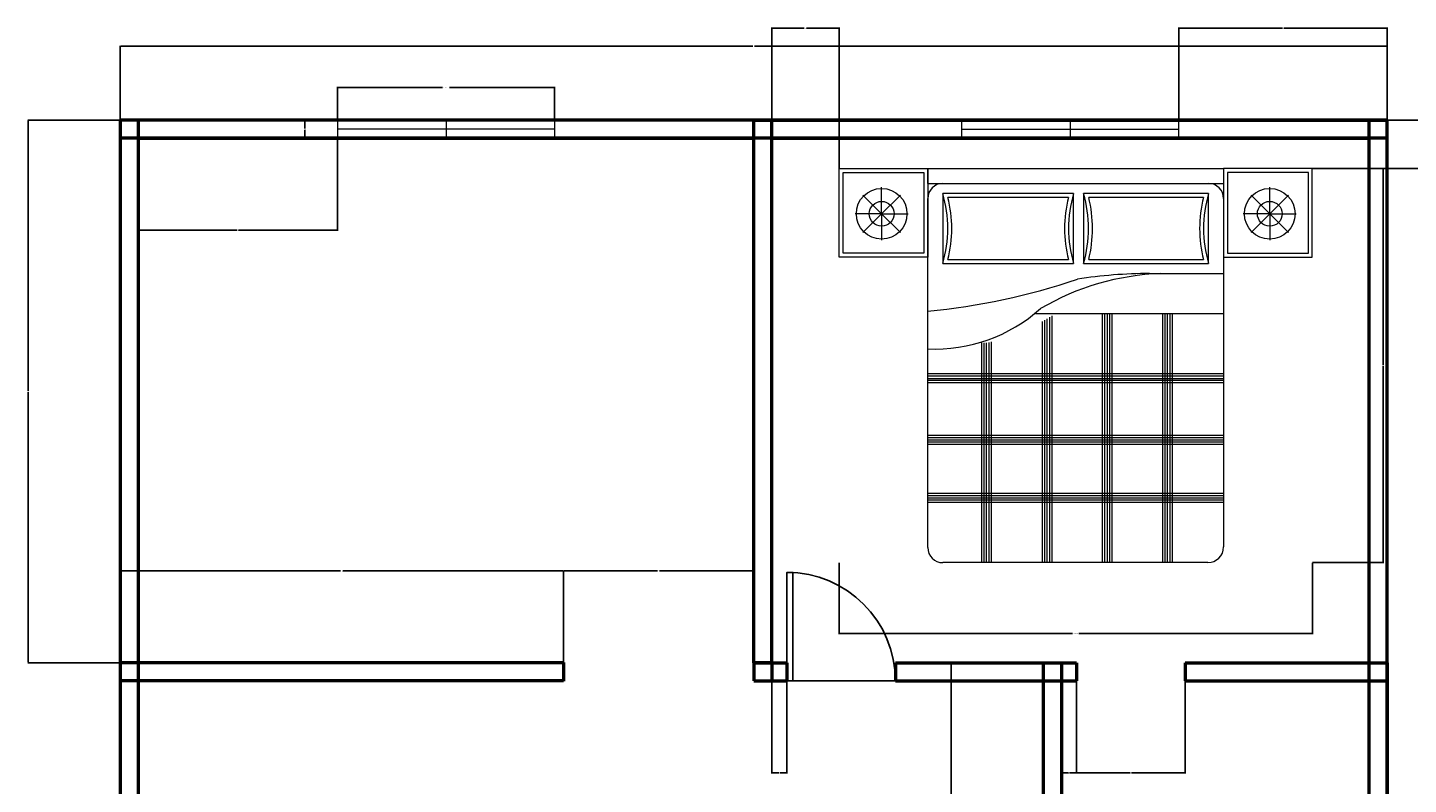
# Model space of a CAD drawing. Units: inches. Extents: x 224 to 929, y 339 to 940.
# Tile 2 of 3: x 224 to 682, y 689 to 940. Entities that reach past the tile are written whole.
import ezdxf

# ---------------------------------------------------------------- set-up
doc = ezdxf.new("R2010")
doc.units = ezdxf.units.IN
for name, color, linetype, lineweight in [('A-ANNO-DIMS', 2, 'Continuous', 18), ('A-DOOR', 3, 'Continuous', 25), ('A-FURN', 8, 'Continuous', 18), ('A-GLAZ', 4, 'Continuous', 18), ('A-WALL', 7, 'Continuous', 50)]:
    doc.layers.add(name, color=color, linetype=linetype, lineweight=lineweight)
doc.styles.get("Standard").update_dxf_attribs({"font": 'arial.ttf'})
doc.dimstyles.get("Standard").update_dxf_attribs({"dimtxt": 0.18, "dimasz": 0.18, "dimexe": 0.18, "dimexo": 0.0625, "dimgap": 0.09, "dimtad": 0, "dimtih": 1, "dimtoh": 1, "dimdec": 4, "dimzin": 0, "dimdsep": 46, "dimtxsty": 'Standard', "dimcen": 0.09, "dimadec": 0, "dimazin": 0, "dimtfac": 1, "dimtdec": 4, "dimtofl": 0, "dimtmove": 0, "dimatfit": 3, "dimfxl": 1, "dimtolj": 1, "dimtzin": 0, "dimarcsym": 0})

# ---------------------------------------------------------------- blocks, each defined once
blk = doc.blocks.new('A$C2EB62172')
at = {"linetype": 'ByBlock'}
for p, q in [((0, 2.0003), (0.45, 2.0003)), ((0, 1.5503), (0, 2.0003)), ((0.45, 1.9241), (0.45, 2.0003)), ((0.45, 2.0003), (0.45, 1.5503)), ((0.45, 2.0003), (1.9506, 2.0003)), ((1.9506, 2.0003), (1.9506, 1.5503)), ((2.4006, 2.0003), (1.9506, 2.0003)), ((2.4006, 1.5503), (2.4006, 2.0003)), ((0.45, 1.9241), (1.9506, 1.9241)), ((0.45, 0.0763), (0.45, 1.8479)), ((1.9506, 1.8479), (1.9506, 0.0801)), ((0.45, 1.5503), (0, 1.5503)), ((1.9506, 1.5503), (2.4006, 1.5503)), ((1.8706, 0.0001), (0.5262, 0.0001))]:
    blk.add_line(p, q, dxfattribs=at)
for p, q in [((0.02, 1.9803), (0.43, 1.9803)), ((0.02, 1.5703), (0.02, 1.9803)), ((0.43, 1.9803), (0.43, 1.5703)), ((1.9706, 1.9803), (1.9706, 1.5703)), ((2.3806, 1.9803), (1.9706, 1.9803)), ((2.3806, 1.5703), (2.3806, 1.9803)), ((0.2161, 1.7703), (0.2161, 1.9047)), ((2.1846, 1.7703), (2.1846, 1.9047)), ((0.2161, 1.7703), (0.1211, 1.8653)), ((0.2161, 1.7703), (0.3111, 1.8653)), ((0.5262, 1.8733), (0.5262, 1.5177)), ((1.1893, 1.8733), (0.5262, 1.8733)), ((1.1632, 1.8533), (0.5523, 1.8533)), ((1.1893, 1.5177), (1.1893, 1.8733)), ((1.2401, 1.8733), (1.2401, 1.5177)), ((1.8744, 1.8733), (1.2401, 1.8733)), ((1.8483, 1.8533), (1.2662, 1.8533)), ((1.8744, 1.5177), (1.8744, 1.8733)), ((2.1846, 1.7703), (2.0896, 1.8653)), ((2.1846, 1.7703), (2.2796, 1.8653)), ((0.2161, 1.7703), (0.0817, 1.7703)), ((0.2161, 1.7703), (0.1211, 1.6753)), ((0.2161, 1.7703), (0.3505, 1.7703)), ((0.2161, 1.7703), (0.3111, 1.6753)), ((0.2161, 1.7703), (0.2161, 1.6359)), ((2.1846, 1.7703), (2.0502, 1.7703)), ((2.1846, 1.7703), (2.0896, 1.6753)), ((2.1846, 1.7703), (2.1846, 1.6359)), ((2.1846, 1.7703), (2.319, 1.7703)), ((2.1846, 1.7703), (2.2796, 1.6753)), ((0.43, 1.5703), (0.02, 1.5703)), ((1.9706, 1.5703), (2.3806, 1.5703)), ((0.5262, 1.5177), (1.1893, 1.5177)), ((0.5523, 1.5377), (1.1632, 1.5377)), ((1.2401, 1.5177), (1.8744, 1.5177)), ((1.2662, 1.5377), (1.8483, 1.5377)), ((1.5747, 1.4669), (1.9506, 1.4669)), ((0.996, 1.2637), (1.9506, 1.2637)), ((1.3351, 1.2637), (1.3351, 0.0001)), ((1.3471, 1.2637), (1.3471, 0.0001)), ((1.3591, 1.2637), (1.3591, 0.0001)), ((1.3722, 1.2637), (1.3722, 0.0001)), ((1.3842, 1.2637), (1.3842, 0.0001)), ((1.6409, 1.2637), (1.6409, 0.0001)), ((1.6529, 1.2637), (1.6529, 0.0001)), ((1.6649, 1.2637), (1.6649, 0.0001)), ((1.678, 1.2637), (1.678, 0.0001)), ((1.69, 1.2637), (1.69, 0.0001)), ((1.0299, 1.2232), (1.0299, 0.0001)), ((1.0419, 1.2301), (1.0419, 0.0001)), ((1.0539, 1.2373), (1.0539, 0.0001)), ((1.067, 1.2453), (1.067, 0.0001)), ((1.079, 1.2529), (1.079, 0.0001)), ((0.722, 1.1147), (0.722, 0.0001)), ((0.734, 1.1147), (0.734, 0.0001)), ((0.746, 1.1147), (0.746, 0.0001)), ((0.7591, 1.1172), (0.7591, 0.0001)), ((0.7711, 1.1203), (0.7711, 0.0001)), ((0.45, 0.9593), (1.9506, 0.9593)), ((0.45, 0.9473), (1.9506, 0.9473)), ((0.45, 0.9353), (1.9506, 0.9353)), ((0.45, 0.9259), (1.9506, 0.9259)), ((0.45, 0.9139), (1.9506, 0.9139)), ((0.45, 0.6471), (1.9506, 0.6471)), ((0.45, 0.6351), (1.9506, 0.6351)), ((0.45, 0.6231), (1.9506, 0.6231)), ((0.45, 0.6137), (1.9506, 0.6137)), ((0.45, 0.6017), (1.9506, 0.6017)), ((0.45, 0.3522), (1.9506, 0.3522)), ((0.45, 0.3402), (1.9506, 0.3402)), ((0.45, 0.3282), (1.9506, 0.3282)), ((0.45, 0.3188), (1.9506, 0.3188)), ((0.45, 0.3068), (1.9506, 0.3068))]:
    blk.add_line(p, q)
for centre, radius in [((0.2161, 1.7703), 0.1285), ((2.1846, 1.7703), 0.1285), ((0.2161, 1.7703), 0.0628), ((2.1846, 1.7703), 0.0628)]:
    blk.add_circle(centre, radius)
for centre, radius, start, end in [((0.5262, 1.8479), 0.0762, 90, 180), ((1.8744, 1.8479), 0.0762, 0, 90), ((0.5262, 0.0763), 0.0762, 180, 270), ((1.8706, 0.0801), 0.08, 270, 0)]:
    blk.add_arc(centre, radius, start, end, dxfattribs=at)
for centre, radius, start, end in [((-0.0834, 1.6955), 0.635, 343.73979, 16.26021), ((-0.0834, 1.6955), 0.655, 346.05939, 13.94061), ((1.7989, 1.6955), 0.655, 166.05939, 193.94061), ((1.7989, 1.6955), 0.635, 163.73979, 196.26021), ((0.6305, 1.6955), 0.635, 343.73979, 16.26021), ((0.6305, 1.6955), 0.655, 346.05939, 13.94061), ((2.484, 1.6955), 0.655, 166.05939, 193.94061), ((2.484, 1.6955), 0.635, 163.73979, 196.26021), ((0.1114, 4.7131), 3.454, 275.6242, 288.5258), ((1.6775, 0.1733), 1.2944, 92.03201, 120.45698), ((1.5739, -0.8648), 2.3317, 89.98016, 99.00664), ((0.4851, 1.8866), 0.8029, 267.49694, 311.91323)]:
    blk.add_arc(centre, radius, start, end)
blk = doc.blocks.new('DOOR-SINGLE-36IN')
blk.add_line((0, 0), (36, 0))
blk.add_lwpolyline([(2, 0), (2, 36), (0, 36), (0, 0)], close=True)
blk.add_arc((0, 0), 36, 0, 90)
blk = doc.blocks.new('WIN-72IN')
for p, q in [((0, 0), (0, 6)), ((36, 0), (36, 6)), ((72, 0), (72, 6)), ((0, 3), (72, 3))]:
    blk.add_line(p, q)
blk = doc.blocks.new('*D7')
at = {"layer": 'A-ANNO-DIMS', "color": 0, "lineweight": -2, "transparency": 16777216}
for p, q in [((326.67, 909.69), (326.67, 920.61)), ((326.85, 920.43), (361.55, 920.43)), ((398.49, 920.43), (363.78, 920.43)), ((398.67, 909.69), (398.67, 920.61))]:
    blk.add_line(p, q, dxfattribs=at)
at = {"layer": 'A-ANNO-DIMS', "color": 0, "transparency": 16777216}
for points in [[(326.85, 920.46), (326.85, 920.4), (326.67, 920.43)], [(398.49, 920.46), (398.49, 920.4), (398.67, 920.43)]]:
    blk.add_solid(points, dxfattribs=at)
at = {"layer": 'Defpoints', "color": 0, "transparency": 16777216}
for p in [(326.67, 920.43), (326.67, 909.63), (398.67, 909.63)]:
    blk.add_point(p, dxfattribs=at)
at = {"layer": 'A-ANNO-DIMS', "color": 0, "transparency": 16777216, "insert": (362.67, 920.43), "char_height": 0.18, "attachment_point": 5}
blk.add_mtext('\\A1;WINDOW 72 TYP.', dxfattribs=at)
blk = doc.blocks.new('*D8')
at = {"layer": 'A-ANNO-DIMS', "color": 0, "lineweight": -2, "transparency": 16777216}
for p, q in [((326.6, 909.63), (315.69, 909.63)), ((315.87, 909.45), (315.87, 906.81)), ((315.87, 903.81), (315.87, 906.44)), ((326.6, 903.63), (315.69, 903.63))]:
    blk.add_line(p, q, dxfattribs=at)
at = {"layer": 'A-ANNO-DIMS', "color": 0, "transparency": 16777216}
for points in [[(315.84, 909.45), (315.9, 909.45), (315.87, 909.63)], [(315.84, 903.81), (315.9, 903.81), (315.87, 903.63)]]:
    blk.add_solid(points, dxfattribs=at)
at = {"layer": 'Defpoints', "color": 0, "transparency": 16777216}
for p in [(326.67, 909.63), (315.87, 903.63), (326.67, 903.63)]:
    blk.add_point(p, dxfattribs=at)
at = {"layer": 'A-ANNO-DIMS', "color": 0, "transparency": 16777216, "insert": (315.87, 906.63), "char_height": 0.18, "attachment_point": 5}
blk.add_mtext('\\A1;6 TYP.', dxfattribs=at)
blk = doc.blocks.new('*D9')
at = {"layer": 'A-ANNO-DIMS', "color": 0, "lineweight": -2, "transparency": 16777216}
for p, q in [((492.98, 762.8), (492.98, 739.15)), ((649.88, 762.8), (649.88, 739.15)), ((493.16, 739.33), (570.35, 739.33)), ((649.7, 739.33), (572.5, 739.33))]:
    blk.add_line(p, q, dxfattribs=at)
at = {"layer": 'A-ANNO-DIMS', "color": 0, "transparency": 16777216}
for points in [[(493.16, 739.36), (493.16, 739.3), (492.98, 739.33)], [(649.7, 739.36), (649.7, 739.3), (649.88, 739.33)]]:
    blk.add_solid(points, dxfattribs=at)
at = {"layer": 'Defpoints', "color": 0, "transparency": 16777216}
for p in [(492.98, 762.86), (649.88, 762.86), (649.88, 739.33)]:
    blk.add_point(p, dxfattribs=at)
at = {"layer": 'A-ANNO-DIMS', "color": 0, "transparency": 16777216, "insert": (571.43, 739.33), "char_height": 0.18, "attachment_point": 5}
blk.add_mtext('\\A1;BED GROUP 157', dxfattribs=at)
blk = doc.blocks.new('*D10')
at = {"layer": 'A-ANNO-DIMS', "color": 0, "lineweight": -2, "transparency": 16777216}
for p, q in [((649.94, 893.59), (673.59, 893.59)), ((673.41, 893.41), (673.41, 828.41)), ((673.41, 763.04), (673.41, 828.05)), ((649.94, 762.86), (673.59, 762.86))]:
    blk.add_line(p, q, dxfattribs=at)
at = {"layer": 'A-ANNO-DIMS', "color": 0, "transparency": 16777216}
for points in [[(673.38, 893.41), (673.44, 893.41), (673.41, 893.59)], [(673.38, 763.04), (673.44, 763.04), (673.41, 762.86)]]:
    blk.add_solid(points, dxfattribs=at)
at = {"layer": 'Defpoints', "color": 0, "transparency": 16777216}
for p in [(649.88, 893.59), (673.41, 893.59), (649.88, 762.86)]:
    blk.add_point(p, dxfattribs=at)
at = {"layer": 'A-ANNO-DIMS', "color": 0, "transparency": 16777216, "insert": (673.41, 828.23), "char_height": 0.18, "attachment_point": 5}
blk.add_mtext('\\A1;131', dxfattribs=at)
blk = doc.blocks.new('*D15')
at = {"layer": 'A-ANNO-DIMS', "color": 0, "lineweight": -2, "transparency": 16777216}
for p, q in [((254.67, 903.69), (254.67, 934.31)), ((254.85, 934.13), (464.37, 934.13)), ((674.49, 934.13), (464.96, 934.13)), ((674.67, 903.69), (674.67, 934.31))]:
    blk.add_line(p, q, dxfattribs=at)
at = {"layer": 'A-ANNO-DIMS', "color": 0, "transparency": 16777216}
for points in [[(254.85, 934.16), (254.85, 934.1), (254.67, 934.13)], [(674.49, 934.16), (674.49, 934.1), (674.67, 934.13)]]:
    blk.add_solid(points, dxfattribs=at)
at = {"layer": 'Defpoints', "color": 0, "transparency": 16777216}
for p in [(674.67, 934.13), (254.67, 903.63), (674.67, 903.63)]:
    blk.add_point(p, dxfattribs=at)
at = {"layer": 'A-ANNO-DIMS', "color": 0, "transparency": 16777216, "insert": (464.67, 934.13), "char_height": 0.18, "attachment_point": 5}
blk.add_mtext('\\A1;420', dxfattribs=at)
blk = doc.blocks.new('*D16')
at = {"layer": 'A-ANNO-DIMS', "color": 0, "lineweight": -2, "transparency": 16777216}
for p, q in [((668.73, 909.63), (699.35, 909.63)), ((699.17, 909.45), (699.17, 639.81)), ((699.17, 369.81), (699.17, 639.44)), ((668.73, 369.63), (699.35, 369.63))]:
    blk.add_line(p, q, dxfattribs=at)
at = {"layer": 'A-ANNO-DIMS', "color": 0, "transparency": 16777216}
for points in [[(699.14, 909.45), (699.2, 909.45), (699.17, 909.63)], [(699.14, 369.81), (699.2, 369.81), (699.17, 369.63)]]:
    blk.add_solid(points, dxfattribs=at)
at = {"layer": 'Defpoints', "color": 0, "transparency": 16777216}
for p in [(668.67, 909.63), (668.67, 369.63), (699.17, 369.63)]:
    blk.add_point(p, dxfattribs=at)
at = {"layer": 'A-ANNO-DIMS', "color": 0, "transparency": 16777216, "insert": (699.17, 639.63), "char_height": 0.18, "attachment_point": 5}
blk.add_mtext('\\A1;540', dxfattribs=at)
blk = doc.blocks.new('*D17')
at = {"layer": 'A-ANNO-DIMS', "color": 0, "lineweight": -2, "transparency": 16777216}
for p, q in [((260.67, 903.56), (260.67, 872.95)), ((326.67, 903.56), (326.67, 872.95)), ((260.85, 873.13), (293.45, 873.13)), ((326.49, 873.13), (293.89, 873.13))]:
    blk.add_line(p, q, dxfattribs=at)
at = {"layer": 'A-ANNO-DIMS', "color": 0, "transparency": 16777216}
for points in [[(260.85, 873.16), (260.85, 873.1), (260.67, 873.13)], [(326.49, 873.16), (326.49, 873.1), (326.67, 873.13)]]:
    blk.add_solid(points, dxfattribs=at)
at = {"layer": 'Defpoints', "color": 0, "transparency": 16777216}
for p in [(260.67, 903.63), (326.67, 903.63), (260.67, 873.13)]:
    blk.add_point(p, dxfattribs=at)
at = {"layer": 'A-ANNO-DIMS', "color": 0, "transparency": 16777216, "insert": (293.67, 873.13), "char_height": 0.18, "attachment_point": 5}
blk.add_mtext('\\A1;66', dxfattribs=at)
blk = doc.blocks.new('*D18')
at = {"layer": 'A-ANNO-DIMS', "color": 0, "lineweight": -2, "transparency": 16777216}
for p, q in [((254.67, 729.69), (254.67, 760.31)), ((254.85, 760.13), (327.73, 760.13)), ((401.39, 760.13), (328.5, 760.13)), ((401.57, 729.69), (401.57, 760.31))]:
    blk.add_line(p, q, dxfattribs=at)
at = {"layer": 'A-ANNO-DIMS', "color": 0, "transparency": 16777216}
for points in [[(254.85, 760.16), (254.85, 760.1), (254.67, 760.13)], [(401.39, 760.16), (401.39, 760.1), (401.57, 760.13)]]:
    blk.add_solid(points, dxfattribs=at)
at = {"layer": 'Defpoints', "color": 0, "transparency": 16777216}
for p in [(401.57, 760.13), (254.67, 729.63), (401.57, 729.63)]:
    blk.add_point(p, dxfattribs=at)
at = {"layer": 'A-ANNO-DIMS', "color": 0, "transparency": 16777216, "insert": (328.12, 760.13), "char_height": 0.18, "attachment_point": 5}
blk.add_mtext('\\A1;146.9', dxfattribs=at)
blk = doc.blocks.new('*D19')
at = {"layer": 'A-ANNO-DIMS', "color": 0, "lineweight": -2, "transparency": 16777216}
for p, q in [((605.67, 909.69), (605.67, 940.31)), ((605.85, 940.13), (639.95, 940.13)), ((674.49, 940.13), (640.39, 940.13)), ((674.67, 909.69), (674.67, 940.31))]:
    blk.add_line(p, q, dxfattribs=at)
at = {"layer": 'A-ANNO-DIMS', "color": 0, "transparency": 16777216}
for points in [[(605.85, 940.16), (605.85, 940.1), (605.67, 940.13)], [(674.49, 940.16), (674.49, 940.1), (674.67, 940.13)]]:
    blk.add_solid(points, dxfattribs=at)
at = {"layer": 'Defpoints', "color": 0, "transparency": 16777216}
for p in [(674.67, 940.13), (605.67, 909.63), (674.67, 909.63)]:
    blk.add_point(p, dxfattribs=at)
at = {"layer": 'A-ANNO-DIMS', "color": 0, "transparency": 16777216, "insert": (640.17, 940.13), "char_height": 0.18, "attachment_point": 5}
blk.add_mtext('\\A1;69', dxfattribs=at)
blk = doc.blocks.new('*D25')
at = {"layer": 'A-ANNO-DIMS', "color": 0, "lineweight": -2, "transparency": 16777216}
for p, q in [((560.6, 729.63), (529.99, 729.63)), ((530.17, 729.45), (530.17, 639.81)), ((530.17, 549.81), (530.17, 639.44)), ((560.6, 549.63), (529.99, 549.63))]:
    blk.add_line(p, q, dxfattribs=at)
at = {"layer": 'A-ANNO-DIMS', "color": 0, "transparency": 16777216}
for points in [[(530.14, 729.45), (530.2, 729.45), (530.17, 729.63)], [(530.14, 549.81), (530.2, 549.81), (530.17, 549.63)]]:
    blk.add_solid(points, dxfattribs=at)
at = {"layer": 'Defpoints', "color": 0, "transparency": 16777216}
for p in [(530.17, 729.63), (560.67, 729.63), (560.67, 549.63)]:
    blk.add_point(p, dxfattribs=at)
at = {"layer": 'A-ANNO-DIMS', "color": 0, "transparency": 16777216, "insert": (530.17, 639.63), "char_height": 0.18, "attachment_point": 5}
blk.add_mtext('\\A1;180', dxfattribs=at)
blk = doc.blocks.new('*D28')
at = {"layer": 'A-ANNO-DIMS', "color": 0, "lineweight": -2, "transparency": 16777216}
for p, q in [((254.6, 909.63), (223.99, 909.63)), ((224.17, 909.45), (224.17, 819.81)), ((224.17, 729.81), (224.17, 819.44)), ((254.6, 729.63), (223.99, 729.63))]:
    blk.add_line(p, q, dxfattribs=at)
at = {"layer": 'A-ANNO-DIMS', "color": 0, "transparency": 16777216}
for points in [[(224.14, 909.45), (224.2, 909.45), (224.17, 909.63)], [(224.14, 729.81), (224.2, 729.81), (224.17, 729.63)]]:
    blk.add_solid(points, dxfattribs=at)
at = {"layer": 'Defpoints', "color": 0, "transparency": 16777216}
for p in [(224.17, 909.63), (254.67, 909.63), (254.67, 729.63)]:
    blk.add_point(p, dxfattribs=at)
at = {"layer": 'A-ANNO-DIMS', "color": 0, "transparency": 16777216, "insert": (224.17, 819.63), "char_height": 0.18, "attachment_point": 5}
blk.add_mtext('\\A1;180', dxfattribs=at)
blk = doc.blocks.new('*D29')
at = {"layer": 'A-ANNO-DIMS', "color": 0, "lineweight": -2, "transparency": 16777216}
for p, q in [((401.57, 729.69), (401.57, 760.31)), ((401.75, 760.13), (432.81, 760.13)), ((464.49, 760.13), (433.43, 760.13)), ((464.67, 729.69), (464.67, 760.31))]:
    blk.add_line(p, q, dxfattribs=at)
at = {"layer": 'A-ANNO-DIMS', "color": 0, "transparency": 16777216}
for points in [[(401.75, 760.16), (401.75, 760.1), (401.57, 760.13)], [(464.49, 760.16), (464.49, 760.1), (464.67, 760.13)]]:
    blk.add_solid(points, dxfattribs=at)
at = {"layer": 'Defpoints', "color": 0, "transparency": 16777216}
for p in [(464.67, 760.13), (401.57, 729.63), (464.67, 729.63)]:
    blk.add_point(p, dxfattribs=at)
at = {"layer": 'A-ANNO-DIMS', "color": 0, "transparency": 16777216, "insert": (433.12, 760.13), "char_height": 0.18, "attachment_point": 5}
blk.add_mtext('\\A1;63.1', dxfattribs=at)
blk = doc.blocks.new('*D31')
at = {"layer": 'A-ANNO-DIMS', "color": 0, "lineweight": -2, "transparency": 16777216}
for p, q in [((571.67, 723.56), (571.67, 692.95)), ((607.67, 723.56), (607.67, 692.95)), ((571.85, 693.13), (589.45, 693.13)), ((607.49, 693.13), (589.88, 693.13))]:
    blk.add_line(p, q, dxfattribs=at)
at = {"layer": 'A-ANNO-DIMS', "color": 0, "transparency": 16777216}
for points in [[(571.85, 693.16), (571.85, 693.1), (571.67, 693.13)], [(607.49, 693.16), (607.49, 693.1), (607.67, 693.13)]]:
    blk.add_solid(points, dxfattribs=at)
at = {"layer": 'Defpoints', "color": 0, "transparency": 16777216}
for p in [(571.67, 723.63), (607.67, 723.63), (571.67, 693.13)]:
    blk.add_point(p, dxfattribs=at)
at = {"layer": 'A-ANNO-DIMS', "color": 0, "transparency": 16777216, "insert": (589.67, 693.13), "char_height": 0.18, "attachment_point": 5}
blk.add_mtext('\\A1;36', dxfattribs=at)
blk = doc.blocks.new('*D32')
at = {"layer": 'A-ANNO-DIMS', "color": 0, "lineweight": -2, "transparency": 16777216}
for p, q in [((566.67, 723.56), (566.67, 692.95)), ((571.67, 723.56), (571.67, 692.95)), ((566.85, 693.13), (569.02, 693.13)), ((571.49, 693.13), (569.32, 693.13))]:
    blk.add_line(p, q, dxfattribs=at)
at = {"layer": 'A-ANNO-DIMS', "color": 0, "transparency": 16777216}
for points in [[(566.85, 693.16), (566.85, 693.1), (566.67, 693.13)], [(571.49, 693.16), (571.49, 693.1), (571.67, 693.13)]]:
    blk.add_solid(points, dxfattribs=at)
at = {"layer": 'Defpoints', "color": 0, "transparency": 16777216}
for p in [(566.67, 723.63), (571.67, 723.63), (566.67, 693.13)]:
    blk.add_point(p, dxfattribs=at)
at = {"layer": 'A-ANNO-DIMS', "color": 0, "transparency": 16777216, "insert": (569.17, 693.13), "char_height": 0.18, "attachment_point": 5}
blk.add_mtext('\\A1;5', dxfattribs=at)
blk = doc.blocks.new('*D33')
at = {"layer": 'A-ANNO-DIMS', "color": 0, "lineweight": -2, "transparency": 16777216}
for p, q in [((470.67, 723.56), (470.67, 692.95)), ((475.67, 723.56), (475.67, 692.95)), ((470.85, 693.13), (473.02, 693.13)), ((475.49, 693.13), (473.32, 693.13))]:
    blk.add_line(p, q, dxfattribs=at)
at = {"layer": 'A-ANNO-DIMS', "color": 0, "transparency": 16777216}
for points in [[(470.85, 693.16), (470.85, 693.1), (470.67, 693.13)], [(475.49, 693.16), (475.49, 693.1), (475.67, 693.13)]]:
    blk.add_solid(points, dxfattribs=at)
at = {"layer": 'Defpoints', "color": 0, "transparency": 16777216}
for p in [(470.67, 723.63), (475.67, 723.63), (470.67, 693.13)]:
    blk.add_point(p, dxfattribs=at)
at = {"layer": 'A-ANNO-DIMS', "color": 0, "transparency": 16777216, "insert": (473.17, 693.13), "char_height": 0.18, "attachment_point": 5}
blk.add_mtext('\\A1;5', dxfattribs=at)
blk = doc.blocks.new('*D36')
at = {"layer": 'A-ANNO-DIMS', "color": 0, "lineweight": -2, "transparency": 16777216}
for p, q in [((470.67, 903.69), (470.67, 940.31)), ((470.85, 940.13), (481.44, 940.13)), ((492.8, 940.13), (482.2, 940.13)), ((492.98, 893.66), (492.98, 940.31))]:
    blk.add_line(p, q, dxfattribs=at)
at = {"layer": 'A-ANNO-DIMS', "color": 0, "transparency": 16777216}
for points in [[(470.85, 940.16), (470.85, 940.1), (470.67, 940.13)], [(492.8, 940.16), (492.8, 940.1), (492.98, 940.13)]]:
    blk.add_solid(points, dxfattribs=at)
at = {"layer": 'Defpoints', "color": 0, "transparency": 16777216}
for p in [(492.98, 940.13), (470.67, 903.63), (492.98, 893.59)]:
    blk.add_point(p, dxfattribs=at)
at = {"layer": 'A-ANNO-DIMS', "color": 0, "transparency": 16777216, "insert": (481.82, 940.13), "char_height": 0.18, "attachment_point": 5}
blk.add_mtext('\\A1;22.31', dxfattribs=at)
blk = doc.blocks.new('*D37')
at = {"layer": 'A-ANNO-DIMS', "color": 0, "lineweight": -2, "transparency": 16777216}
for p, q in [((668.73, 909.63), (705.35, 909.63)), ((705.17, 909.45), (705.17, 901.79)), ((705.17, 893.77), (705.17, 901.43)), ((649.94, 893.59), (705.35, 893.59))]:
    blk.add_line(p, q, dxfattribs=at)
at = {"layer": 'A-ANNO-DIMS', "color": 0, "transparency": 16777216}
for points in [[(705.14, 909.45), (705.2, 909.45), (705.17, 909.63)], [(705.14, 893.77), (705.2, 893.77), (705.17, 893.59)]]:
    blk.add_solid(points, dxfattribs=at)
at = {"layer": 'Defpoints', "color": 0, "transparency": 16777216}
for p in [(668.67, 909.63), (649.88, 893.59), (705.17, 893.59)]:
    blk.add_point(p, dxfattribs=at)
at = {"layer": 'A-ANNO-DIMS', "color": 0, "transparency": 16777216, "insert": (705.17, 901.61), "char_height": 0.18, "attachment_point": 5}
blk.add_mtext('\\A1;16.032', dxfattribs=at)

msp = doc.modelspace()

# ---------------------------------------------------------------- linework, layer by layer
at = {"layer": 'A-WALL'}
for p, q in [((674.6661, 909.6252), (254.6661, 909.6252)), ((254.6661, 909.6252), (254.6661, 465.6252)), ((260.6661, 909.6252), (260.6661, 465.6252)), ((464.6661, 909.6252), (674.6661, 909.6252)), ((464.6661, 729.6252), (464.6661, 909.6252)), ((470.6661, 729.6252), (470.6661, 909.6252)), ((668.6661, 369.6252), (668.6661, 909.6252)), ((674.6661, 369.6252), (674.6661, 909.6252)), ((674.6661, 903.6252), (254.6661, 903.6252)), ((260.6661, 903.6252), (464.6661, 903.6252)), ((470.6661, 903.6252), (668.6661, 903.6252)), ((401.5722, 729.6252), (254.6661, 729.6252)), ((401.5722, 729.6989), (401.5722, 723.5553)), ((464.6661, 729.6252), (475.6661, 729.6252)), ((470.6661, 729.6252), (464.6661, 729.6252)), ((464.6661, 729.6252), (464.6661, 723.6252)), ((470.6661, 729.6252), (470.6661, 723.6252)), ((475.6661, 729.6252), (475.6661, 723.6252)), ((511.6661, 729.6252), (511.6661, 723.6252)), ((511.6661, 729.6252), (571.6661, 729.6252)), ((560.6661, 729.6252), (560.6661, 549.6252)), ((566.6661, 729.6252), (566.6661, 549.6252)), ((566.6661, 729.6252), (566.6661, 723.6252)), ((569.6661, 729.6252), (571.6661, 729.6252)), ((571.6661, 729.6252), (571.6661, 723.6252)), ((607.6661, 729.6252), (607.6661, 723.6252)), ((607.6661, 729.6252), (674.6661, 729.6252)), ((607.6661, 729.6252), (674.6661, 729.6252)), ((674.6661, 729.6252), (674.6661, 549.6252)), ((401.5722, 723.6252), (254.6661, 723.6252)), ((464.6661, 723.6252), (475.6661, 723.6252)), ((511.6661, 723.6252), (571.6661, 723.6252)), ((607.6661, 723.6252), (674.6661, 723.6252))]:
    msp.add_line(p, q, dxfattribs=at)

# ---------------------------------------------------------------- block references
at = {"layer": 'A-DOOR'}
msp.add_blockref('DOOR-SINGLE-36IN', (475.666, 723.625), dxfattribs=at)
at = {"layer": 'A-FURN', "xscale": 65.35814540157314, "yscale": 65.35814540157314, "zscale": 65.35814540157314}
msp.add_blockref('A$C2EB62172', (492.9744, 762.8573), dxfattribs=at)
at = {"layer": 'A-GLAZ', "rotation": 180}
msp.add_blockref('WIN-72IN', (398.6663, 909.6253), dxfattribs=at)
at = {"layer": 'A-GLAZ'}
msp.add_blockref('WIN-72IN', (533.666, 903.625), dxfattribs=at)

# ---------------------------------------------------------------- dimensions: what is measured, and where the dimension line sits
at = {"layer": 'A-ANNO-DIMS'}
for base, p1, p2, override, picture, middle in [((492.9771, 940.1252), (470.6661, 903.6252), (492.9771, 893.5934), {"dimdec": 2, "dimlfac": 1, "dimrnd": 0, "dimzin": 0, "dimdsep": 46, "dimlunit": 2}, '*D36', (481.8216, 940.1252)), ((674.6661, 934.1252), (254.6661, 903.6252), (674.6661, 903.6252), {"dimdec": 0, "dimlfac": 1, "dimrnd": 0, "dimzin": 0, "dimdsep": 46, "dimlunit": 2}, '*D15', (464.6661, 934.1252)), ((464.6661, 760.1252), (401.5722, 729.6252), (464.6661, 729.6252), {"dimdec": 1, "dimlfac": 1, "dimrnd": 0, "dimzin": 0, "dimdsep": 46, "dimlunit": 2}, '*D29', (433.1192, 760.1252))]:
    dim = msp.add_linear_dim(base=base, p1=p1, p2=p2, dimstyle='Standard', override=override, dxfattribs=at)
    dim.commit()
    dim.dimension.update_dxf_attribs({"geometry": picture, "text_midpoint": middle})
for base, p1, p2, angle, override, picture, middle in [((674.6661, 940.1252), (605.6661, 909.6252), (674.6661, 909.6252), 0, {"dimdec": 0, "dimlfac": 1, "dimrnd": 0, "dimzin": 0, "dimdsep": 46, "dimlunit": 2}, '*D19', (640.1661, 940.1252)), ((224.1661, 909.6252), (254.6661, 729.6252), (254.6661, 909.6252), 90, {"dimdec": 0, "dimlfac": 1, "dimrnd": 0, "dimzin": 0, "dimdsep": 46, "dimlunit": 2}, '*D28', (224.1661, 819.6252)), ((705.1661, 893.5934), (668.6661, 909.6252), (649.8759, 893.5934), 90, {"dimdec": 3, "dimlfac": 1, "dimrnd": 0, "dimzin": 0, "dimdsep": 46, "dimlunit": 2}, '*D37', (705.1661, 901.6093)), ((699.1661, 369.6252), (668.6661, 909.6252), (668.6661, 369.6252), 270, {"dimdec": 0, "dimlfac": 1, "dimrnd": 0, "dimzin": 0, "dimdsep": 46, "dimlunit": 2}, '*D16', (699.1661, 639.6252)), ((260.6661, 873.1252), (326.6661, 903.6252), (260.6661, 903.6252), 180, {"dimdec": 0, "dimlfac": 1, "dimrnd": 0, "dimzin": 0, "dimdsep": 46, "dimlunit": 2}, '*D17', (293.6661, 873.1252)), ((673.4107, 893.5934), (649.8759, 762.8641), (649.8759, 893.5934), 90, {"dimdec": 0, "dimlfac": 1, "dimrnd": 0, "dimzin": 0, "dimdsep": 46, "dimlunit": 2}, '*D10', (673.4107, 828.2287)), ((401.5722, 760.1252), (254.6661, 729.6252), (401.5722, 729.6252), 0, {"dimdec": 1, "dimlfac": 1, "dimrnd": 0, "dimzin": 0, "dimdsep": 46, "dimlunit": 2}, '*D18', (328.1192, 760.1252)), ((530.1661, 729.6252), (560.6661, 549.6252), (560.6661, 729.6252), 90, {"dimdec": 0, "dimlfac": 1, "dimrnd": 0, "dimzin": 0, "dimdsep": 46, "dimlunit": 2}, '*D25', (530.1661, 639.6252)), ((470.6661, 693.1252), (475.6661, 723.6252), (470.6661, 723.6252), 180, {"dimdec": 0, "dimlfac": 1, "dimrnd": 0, "dimzin": 0, "dimdsep": 46, "dimlunit": 2}, '*D33', (473.1661, 693.1252)), ((566.6661, 693.1252), (571.6661, 723.6252), (566.6661, 723.6252), 180, {"dimdec": 0, "dimlfac": 1, "dimrnd": 0, "dimzin": 0, "dimdsep": 46, "dimlunit": 2}, '*D32', (569.1661, 693.1252)), ((571.6661, 693.1252), (607.6661, 723.6252), (571.6661, 723.6252), 180, {"dimdec": 0, "dimlfac": 1, "dimrnd": 0, "dimzin": 0, "dimdsep": 46, "dimlunit": 2}, '*D31', (589.6661, 693.1252))]:
    dim = msp.add_linear_dim(base=base, p1=p1, p2=p2, angle=angle, dimstyle='Standard', override=override, dxfattribs=at)
    dim.commit()
    dim.dimension.update_dxf_attribs({"geometry": picture, "text_midpoint": middle})
for base, p1, p2, angle, text, picture, middle in [((326.6661, 920.4252), (398.6661, 909.6252), (326.6661, 909.6252), 180, 'WINDOW <> TYP.', '*D7', (362.6661, 920.4252)), ((315.8661, 903.6252), (326.6661, 909.6252), (326.6661, 903.6252), 270, '<> TYP.', '*D8', (315.8661, 906.6252))]:
    dim = msp.add_linear_dim(base=base, p1=p1, p2=p2, angle=angle, text=text, dimstyle='Standard', override={"dimdec": 0, "dimlfac": 1, "dimrnd": 0, "dimzin": 0, "dimdsep": 46, "dimlunit": 2}, dxfattribs=at)
    dim.commit()
    dim.dimension.update_dxf_attribs({"geometry": picture, "text_midpoint": middle})
dim = msp.add_linear_dim(base=(649.8759, 739.3292), p1=(492.9771, 762.8641), p2=(649.8759, 762.8641), text='BED GROUP <>', dimstyle='Standard', override={"dimdec": 0, "dimlfac": 1, "dimrnd": 0, "dimzin": 0, "dimdsep": 46, "dimlunit": 2}, dxfattribs=at)
dim.commit()
dim.dimension.update_dxf_attribs({"geometry": '*D9', "text_midpoint": (571.4265, 739.3292)})

doc.saveas('drawing.dxf')
